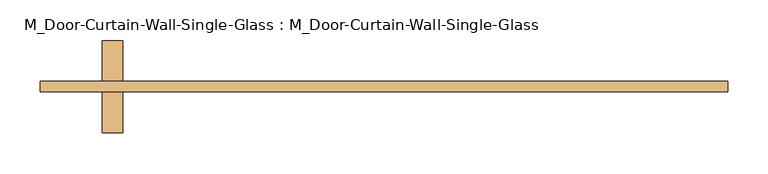
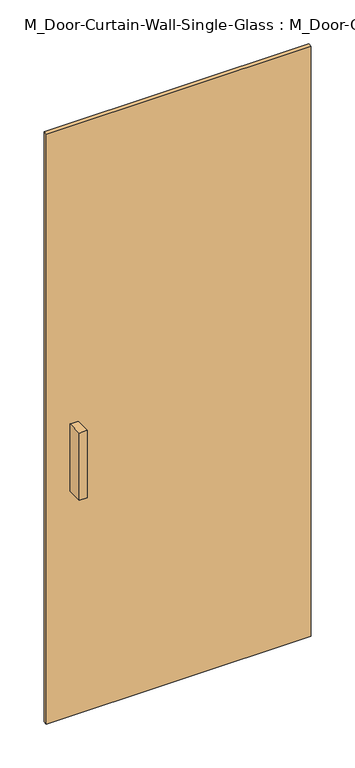
"""IFC4 building model written with IfcOpenShell, lengths in millimetres: door geometry, M_Door-Curtain-Wall-Single-Glass : M_Door-Curtain-Wall-Single-Glass."""

from ifc_helpers import new_model, si_unit, frame, origin, origin_with_axes, place, context, project, spatial, polyline, outline, extrude, source, transform, mapped, element, save


def m_door_curtain_wall_single_glass_m_door_curtain_wall_single_f8ee2cb8(model_context):
    return source(origin(), model_context, "Body", "SweptSolid", [
        extrude(outline(polyline([(425.0, 50.8), (425.0, 38.1), (-425.0, 38.1), (-425.0, 50.8), (425.0, 50.8)])), origin_with_axes(), (0.0, 0.0, 1.0), 2000.0),
        extrude(outline(polyline([(-348.8, 101.6), (-323.4, 101.6), (-323.4, 50.8), (-348.8, 50.8), (-348.8, 101.6)])), frame((0.0, 0.0, 762.0), z_axis=(0.0, 0.0, 1.0), x_axis=(1.0, 0.0, 0.0)), (0.0, 0.0, 1.0), 228.6),
        extrude(outline(polyline([(-323.4, -12.7), (-348.8, -12.7), (-348.8, 38.1), (-323.4, 38.1), (-323.4, -12.7)])), frame((0.0, 0.0, 762.0), z_axis=(0.0, 0.0, 1.0), x_axis=(1.0, 0.0, 0.0)), (0.0, 0.0, 1.0), 228.6),
    ])


if __name__ == "__main__":
    model = new_model("IFC4")
    model_context = context("Model", 3, world=origin())
    ifc_project = project(units=[si_unit("LENGTHUNIT", "METRE", prefix="MILLI")], contexts=[model_context])
    site = spatial("IfcSite", under=ifc_project)
    building = spatial("IfcBuilding", under=site)
    placement = place(None, origin())
    m_door_curtain_wall_single_glass_m_door_curtain_wall_single_shape = m_door_curtain_wall_single_glass_m_door_curtain_wall_single_f8ee2cb8(model_context)
    element("IfcDoor", 1, ObjectType="M_Door-Curtain-Wall-Single-Glass : M_Door-Curtain-Wall-Single-Glass", at=placement, inside=building, context=model_context, shape_type="MappedRepresentation", body=[
        mapped(m_door_curtain_wall_single_glass_m_door_curtain_wall_single_shape, transform((0.0, 0.0, 0.0), x_axis=(1.0, 0.0, 0.0), y_axis=(0.0, 1.0, 0.0), z_axis=(0.0, 0.0, 1.0))),
    ])
    save(model, "model.ifc")

# Revit data of these elements
# Type "M_Door-Curtain-Wall-Single-Glass : M_Door-Curtain-Wall-Single-Glass"
#   Type Mark = "51"
#   Assembly Code = "B2030100"
#   Analytic Construction = "<None>"
#   Width [instance default] = 900 mm
#   Thermal Resistance (R) = 1.7611 (m²·K)/W
#   Swing Angle [instance default] = 90.00°
#   Heat Transfer Coefficient (U) = 0.567826 W/(m²·K)
#   Offset = 50.8 mm
#   Define Thermal Properties by = 1
#   Function = 1
#   Door Handle Material = Aluminum
#   Glazing = Glass
#   Visual Light Transmittance = 0
#   Solar Heat Gain Coefficient = 0
#   Construction Type Id = ""
# Element 1 (IfcDoor, "M_Door-Curtain-Wall-Single-Glass : M_Door-Curtain-Wall-Single-Glass")
#   Width = 850 mm
#   Materials on its faces: "Aluminum", "Glass"
# Materials
#   "Aluminum": class "Metal", colour RGB 247 247 247, transparency 0, Description = "Aluminum 6061", Cost = 0
#   "Glass": class "Glass", colour RGB 0 128 192, transparency 0.9, Description = "Soda Lime Glass", Cost = 0
